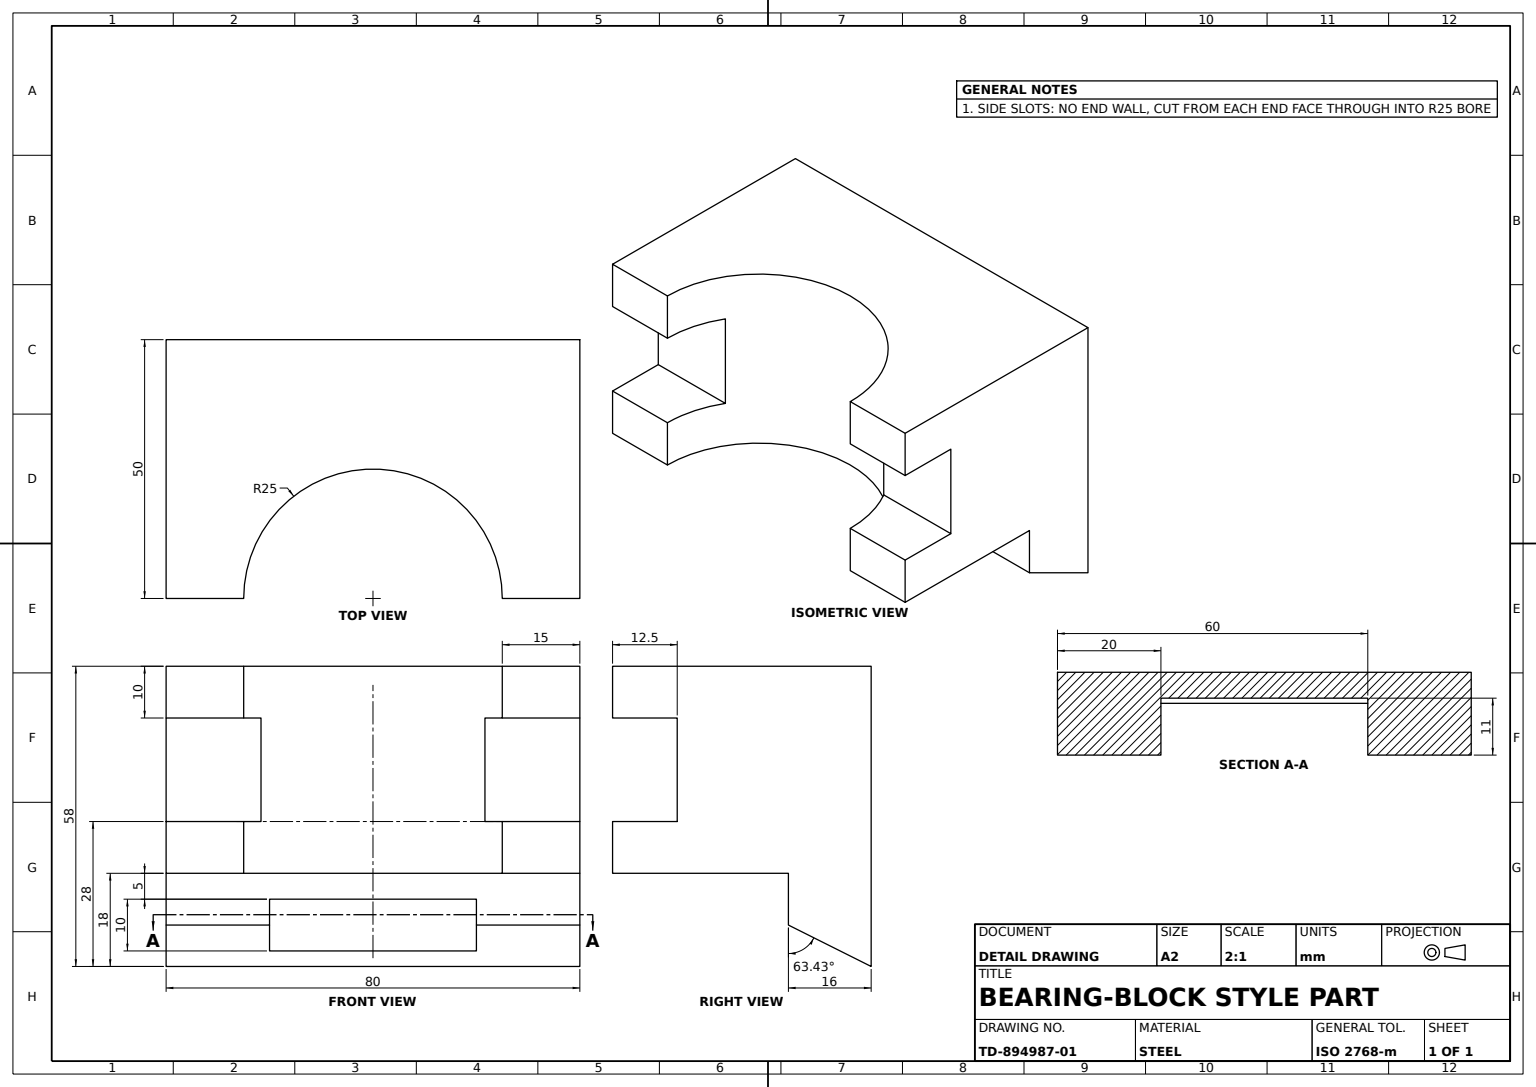
from build123d import *

# Parameters (mm, degrees)
BASE_BLOCK_SKETCH_W        = 80
BASE_BLOCK_SKETCH_H        = 58
BASE_BLOCK_DEPTH           = 16
UPPER_BLOCK_DEPTH          = 10
SIDE_BLOCK_80_DEPTH        = 80
SEMICIRCULAR_BORE_50_DEPTH = 30
RECTANGULAR_SLOT_SKETCH_W  = 43.30127019
RECTANGULAR_SLOT_SKETCH_H  = 12.5
RECTANGULAR_SLOT_DEPTH     = 10
BORE_SIDE_GROOVES_DEPTH    = 10
WEDGE_CUT_DEPTH            = 80
BOTTOM_NOTCH_DEPTH         = 11


with BuildPart() as part:
    # Base Block Sketch → Base Block (new body)
    with BuildSketch(Plane.XY):
        with Locations((40, -29)):
            Rectangle(BASE_BLOCK_SKETCH_W, BASE_BLOCK_SKETCH_H)
    extrude(amount=BASE_BLOCK_DEPTH)

    # Upper Block Sketch → Upper Block (add)
    with BuildSketch(Plane(origin=(0, 0, 0), x_dir=(1, 0, 0), z_dir=(0, 1, 0))):
        with BuildLine():
            Line((0, -16), (0, -50))
            Line((0, -50), (15, -50))
            ThreePointArc((15, -50), (40, -25), (65, -50))
            Line((65, -50), (80, -50))
            Line((80, -50), (80, -16))
            Line((80, -16), (0, -16))
        make_face()
    extrude(amount=-UPPER_BLOCK_DEPTH)

    # Side Block Sketch → Side Block 80 (add)
    with BuildSketch(Plane.ZY):
        Polygon((37.5, -10), (37.5, -30), (50, -30), (50, -40), (16, -40), (16, -10), align=None)
    extrude(amount=-SIDE_BLOCK_80_DEPTH)

    # Bore Ø50 Sketch → Semicircular Bore Ø50 (cut)
    with BuildSketch(Plane(origin=(0, -10, 0), x_dir=(1, 0, 0), z_dir=(0, 1, 0))):
        with BuildLine():
            Line((18.349364905, -37.5), (61.650635095, -37.5))
            ThreePointArc((61.650635095, -37.5), (40, -25), (18.349364905, -37.5))
        make_face()
    extrude(amount=-SEMICIRCULAR_BORE_50_DEPTH, mode=Mode.SUBTRACT)

    # Rectangular Slot Sketch → Rectangular Slot (cut)
    with BuildSketch(Plane.XZ.offset(40)):
        with Locations((40, 43.75)):
            Rectangle(RECTANGULAR_SLOT_SKETCH_W, RECTANGULAR_SLOT_SKETCH_H)
    extrude(amount=-RECTANGULAR_SLOT_DEPTH, mode=Mode.SUBTRACT)

    # Bore Grooves Sketch → Bore Side Grooves (cut)
    with BuildSketch(Plane(origin=(0, -30, 0), x_dir=(1, 0, 0), z_dir=(0, 1, 0))):
        with BuildLine():
            Line((15, -50), (18.349364905, -50))
            Line((18.349364905, -50), (18.349364905, -37.5))
            ThreePointArc((18.349364905, -37.5), (15.851854343, -43.529523872), (15, -50))
        make_face()
        with BuildLine():
            Line((65, -50), (61.650635095, -50))
            Line((61.650635095, -50), (61.650635095, -37.5))
            ThreePointArc((61.650635095, -37.5), (64.148145657, -43.529523872), (65, -50))
        make_face()
    extrude(amount=-BORE_SIDE_GROOVES_DEPTH, mode=Mode.SUBTRACT)

    # Wedge Cut Sketch → Wedge Cut (cut)
    with BuildSketch(Plane.ZY):
        Polygon((16, -50), (0, -58), (16, -58), align=None)
    extrude(amount=-WEDGE_CUT_DEPTH, mode=Mode.SUBTRACT)

    # Bottom Notch Sketch → Bottom Notch (cut)
    with BuildSketch(Plane.XY.offset(16)):
        Polygon((60, -50), (60, -45), (20, -45), (20, -55), (60, -55), align=None)
    extrude(amount=-BOTTOM_NOTCH_DEPTH, mode=Mode.SUBTRACT)


solid = part.part
